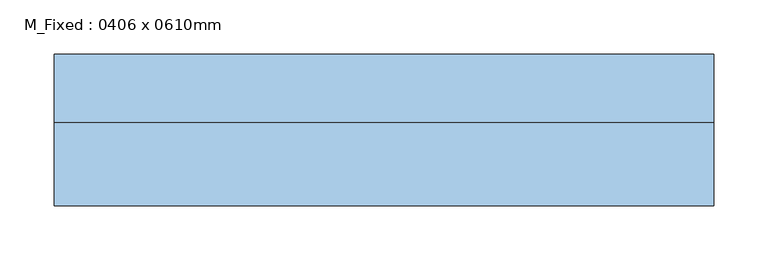
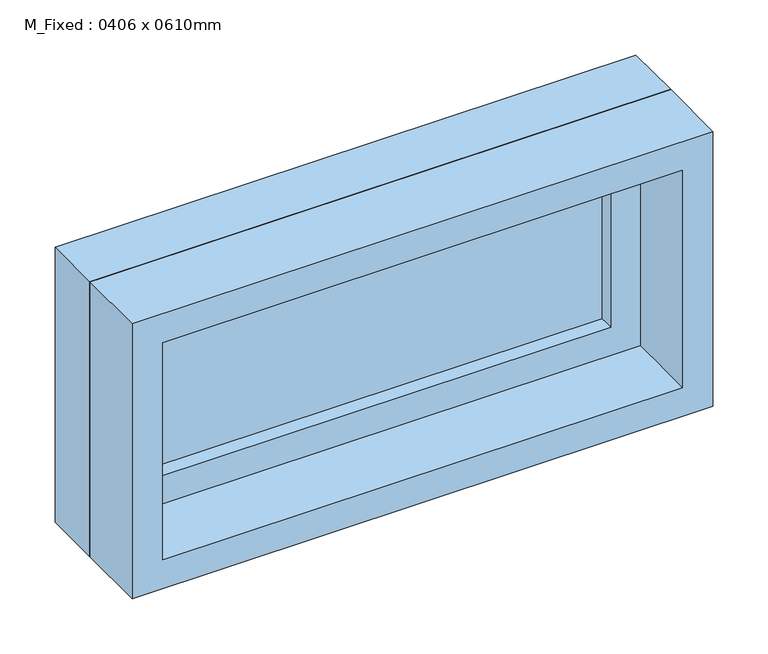
"""IFC4 building model written with IfcOpenShell, lengths in millimetres: window geometry, M_Fixed : 0406 x 0610mm."""

from ifc_helpers import new_model, si_unit, frame, origin, place, context, project, spatial, polyline, outline, extrude, source, transform, mapped, element, save


def m_fixed_0406_x_0610mm_8d3231a3(model_context):
    return source(origin(), model_context, "Body", "SweptSolid", [
        extrude(outline(polyline([(-241.8, 48.0), (241.8, 48.0), (241.8, 36.0), (-241.8, 36.0), (-241.8, 48.0)])), frame((0.0, 0.0, 978.0), z_axis=(0.0, 0.0, 1.0), x_axis=(1.0, 0.0, 0.0)), (0.0, 0.0, 1.0), 178.8),
        extrude(outline(polyline([(1200.8, -285.8), (934.0, -285.8), (934.0, 285.8), (1200.8, 285.8), (1200.8, -285.8)]), holes=[polyline([(1156.8, -241.8), (1156.8, 241.8), (978.0, 241.8), (978.0, -241.8), (1156.8, -241.8)])]), frame((0.0, 20.0, 0.0), z_axis=(0.0, 1.0, 0.0), x_axis=(0.0, 0.0, 1.0)), (0.0, 0.0, 1.0), 44.0),
        extrude(outline(polyline([(1219.8, -304.8), (915.0, -304.8), (915.0, 304.8), (1219.8, 304.8), (1219.8, -304.8)]), holes=[polyline([(1200.8, -285.8), (1200.8, 285.8), (934.0, 285.8), (934.0, -285.8), (1200.8, -285.8)])]), frame((0.0, 20.0, 0.0), z_axis=(0.0, 1.0, 0.0), x_axis=(0.0, 0.0, 1.0)), (0.0, 0.0, 1.0), 63.0),
        extrude(outline(polyline([(1219.8, -304.8), (915.0, -304.8), (915.0, 304.8), (1219.8, 304.8), (1219.8, -304.8)]), holes=[polyline([(1187.8, -272.8), (1187.8, 272.8), (947.0, 272.8), (947.0, -272.8), (1187.8, -272.8)])]), frame((0.0, -57.0, 0.0), z_axis=(0.0, 1.0, 0.0), x_axis=(0.0, 0.0, 1.0)), (0.0, 0.0, 1.0), 77.0),
    ])


if __name__ == "__main__":
    model = new_model("IFC4")
    model_context = context("Model", 3, world=origin())
    ifc_project = project(units=[si_unit("LENGTHUNIT", "METRE", prefix="MILLI")], contexts=[model_context])
    site = spatial("IfcSite", under=ifc_project)
    building = spatial("IfcBuilding", under=site)
    placement = place(None, origin())
    m_fixed_0406_x_0610mm_shape = m_fixed_0406_x_0610mm_8d3231a3(model_context)
    element("IfcWindow", 1, ObjectType="M_Fixed : 0406 x 0610mm", at=placement, inside=building, context=model_context, shape_type="MappedRepresentation", body=[
        mapped(m_fixed_0406_x_0610mm_shape, transform((0.0, 0.0, 0.0), x_axis=(1.0, 0.0, 0.0), y_axis=(0.0, 1.0, 0.0), z_axis=(0.0, 0.0, 1.0))),
    ])
    save(model, "model.ifc")

# Revit data of these elements
# Type "M_Fixed : 0406 x 0610mm"
#   Type Mark = "10"
#   Construction Type Id = "GSP4R"
#   Analytic Construction = "1/8 in Pilkington single glazing"
#   Visual Light Transmittance = 0.9
#   Thermal Resistance (R) = 0.271106 (m²·K)/W
#   Solar Heat Gain Coefficient = 0.78
#   Heat Transfer Coefficient (U) = 3.6886 W/(m²·K)
#   Height = 1 ft
#   Default Sill Height = 3.001969 ft
#   Width = 2 ft
#   Window Inset = 0.062336 ft
#   Define Thermal Properties by = 1
#   Define Thermal Properties by = 1
#   Frame Exterior Material = Sash
#   Frame Interior Material = Sash
#   Glass Pane Material = Glass
#   Sash = Sash
#   Wall Closure = (empty or 0)
# Element 1 (IfcWindow, "M_Fixed : 0406 x 0610mm")
#   Materials on its faces: "Sash", "Glass"
# Materials
#   "Sash": class "Wood", colour RGB 224 178 126, transparency 0, Cost = 0
#   "Glass": class "Glass", colour RGB 0 128 192, transparency 0.9, Description = "Soda Lime Glass", Cost = 0
